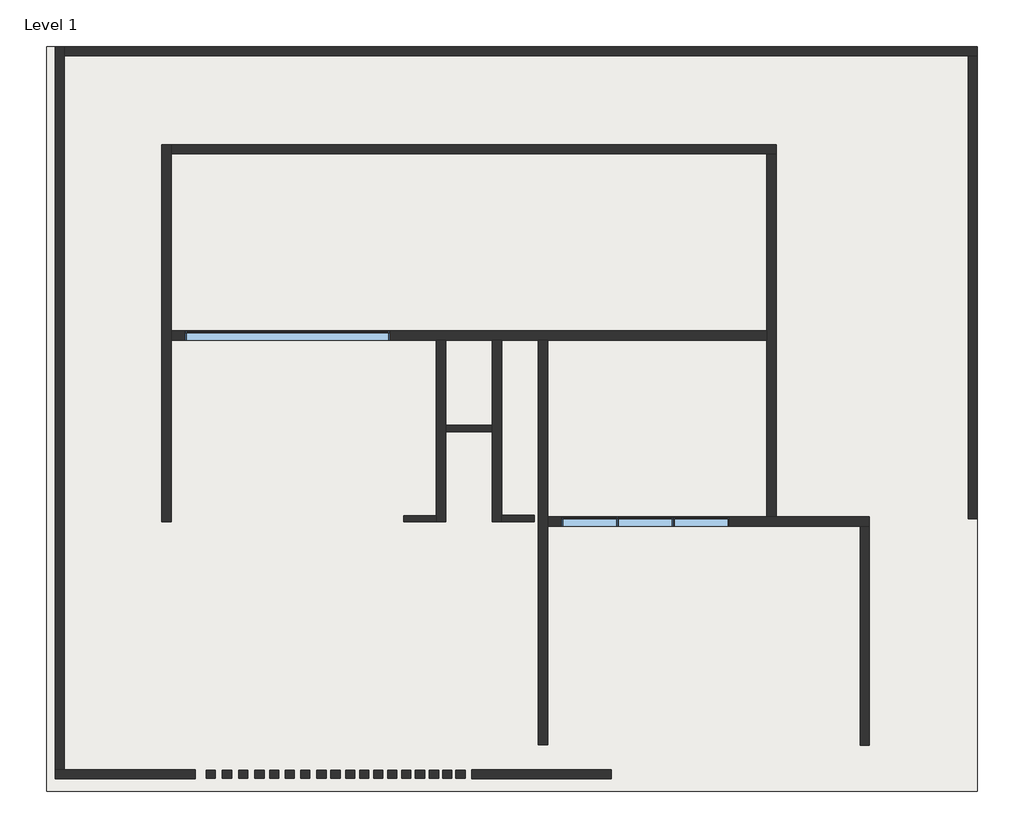
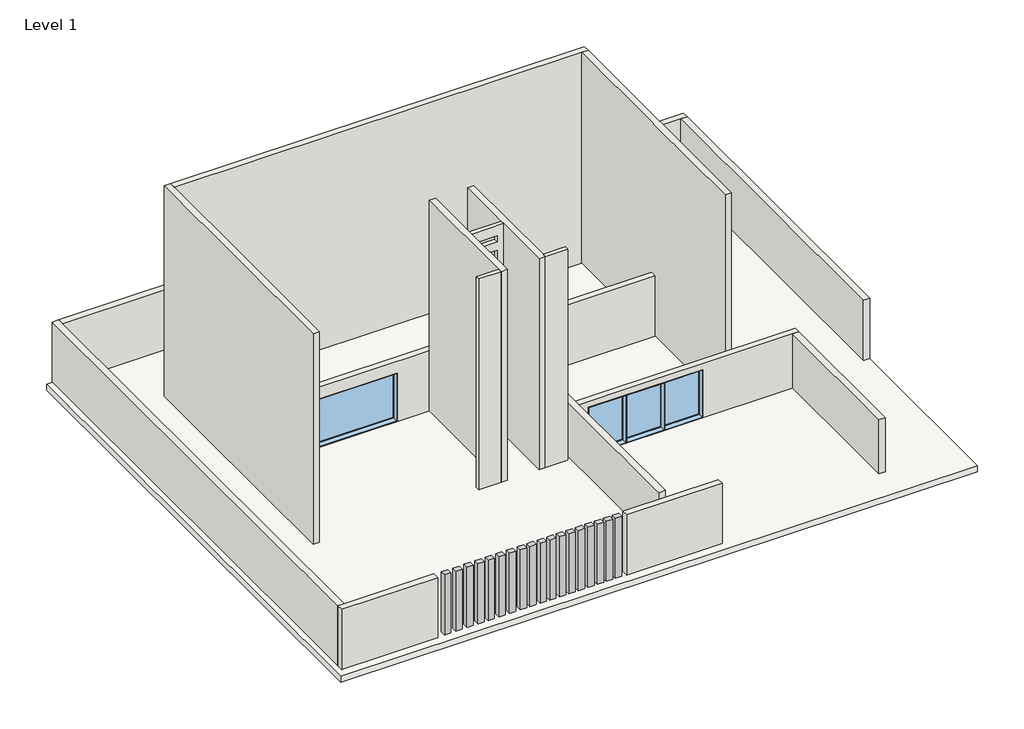
# One storey: 18 columns, 17 walls, 4 windows, 1 slab.
"""IFC4 building model written with IfcOpenShell, lengths in millimetres."""

from ifc_helpers import new_model, si_unit, frame, origin, origin_with_axes, place, context, project, spatial, polyline, outline, extrude, faceted_brep, transform, mapped, element, save
from components import column_263bc08f, window_e4c9328c, window_1de08d8e

model = new_model("IFC4")

# Units and contexts
model_context = context("Model", 3, world=origin())
ifc_project = project(units=[si_unit("LENGTHUNIT", "METRE", prefix="MILLI")], contexts=[model_context])

# Site, building, storey
site = spatial("IfcSite", under=ifc_project)
building = spatial("IfcBuilding", under=site)
storey = spatial("IfcBuildingStorey", under=building, Name="Level 1", Elevation=0.0)

# Columns
placement = place(None, origin())
column_shape = column_263bc08f(model_context)
element("IfcColumn", 1, ObjectType="Rectangular Column : 18\" x 18\"", at=placement, inside=storey, context=model_context, shape_type="MappedRepresentation", body=[
    mapped(column_shape, transform((-8214.6338476, -8321.9583832, 0.0), x_axis=(1.0, 0.0, 0.0), y_axis=(0.0, 1.0, 0.0), z_axis=(0.0, 0.0, 1.0))),
])
element("IfcColumn", 2, ObjectType="Rectangular Column : 18\" x 18\"", at=placement, inside=storey, context=model_context, shape_type="MappedRepresentation", body=[
    mapped(column_shape, transform((-8646.4338476, -8321.9583832, 0.0), x_axis=(1.0, 0.0, 0.0), y_axis=(0.0, 1.0, 0.0), z_axis=(0.0, 0.0, 1.0))),
])
element("IfcColumn", 3, ObjectType="Rectangular Column : 18\" x 18\"", at=placement, inside=storey, context=model_context, shape_type="MappedRepresentation", body=[
    mapped(column_shape, transform((-9078.2338476, -8321.9583832, 0.0), x_axis=(1.0, 0.0, 0.0), y_axis=(0.0, 1.0, 0.0), z_axis=(0.0, 0.0, 1.0))),
])
element("IfcColumn", 4, ObjectType="Rectangular Column : 18\" x 18\"", at=placement, inside=storey, context=model_context, shape_type="MappedRepresentation", body=[
    mapped(column_shape, transform((-9535.4338476, -8321.9583832, 0.0), x_axis=(1.0, 0.0, 0.0), y_axis=(0.0, 1.0, 0.0), z_axis=(0.0, 0.0, 1.0))),
])
element("IfcColumn", 5, ObjectType="Rectangular Column : 18\" x 18\"", at=placement, inside=storey, context=model_context, shape_type="MappedRepresentation", body=[
    mapped(column_shape, transform((-9992.6338476, -8321.9583832, 0.0), x_axis=(1.0, 0.0, 0.0), y_axis=(0.0, 1.0, 0.0), z_axis=(0.0, 0.0, 1.0))),
])
element("IfcColumn", 6, ObjectType="Rectangular Column : 18\" x 18\"", at=placement, inside=storey, context=model_context, shape_type="MappedRepresentation", body=[
    mapped(column_shape, transform((-10449.8338476, -8321.9583832, 0.0), x_axis=(1.0, 0.0, 0.0), y_axis=(0.0, 1.0, 0.0), z_axis=(0.0, 0.0, 1.0))),
])
element("IfcColumn", 7, ObjectType="Rectangular Column : 18\" x 18\"", at=placement, inside=storey, context=model_context, shape_type="MappedRepresentation", body=[
    mapped(column_shape, transform((-10907.0338476, -8321.9583832, 0.0), x_axis=(1.0, 0.0, 0.0), y_axis=(0.0, 1.0, 0.0), z_axis=(0.0, 0.0, 1.0))),
])
element("IfcColumn", 8, ObjectType="Rectangular Column : 18\" x 18\"", at=placement, inside=storey, context=model_context, shape_type="MappedRepresentation", body=[
    mapped(column_shape, transform((-11364.2338476, -8321.9583832, 0.0), x_axis=(1.0, 0.0, 0.0), y_axis=(0.0, 1.0, 0.0), z_axis=(0.0, 0.0, 1.0))),
])
element("IfcColumn", 9, ObjectType="Rectangular Column : 18\" x 18\"", at=placement, inside=storey, context=model_context, shape_type="MappedRepresentation", body=[
    mapped(column_shape, transform((-11821.4338476, -8321.9583832, 0.0), x_axis=(1.0, 0.0, 0.0), y_axis=(0.0, 1.0, 0.0), z_axis=(0.0, 0.0, 1.0))),
])
element("IfcColumn", 10, ObjectType="Rectangular Column : 18\" x 18\"", at=placement, inside=storey, context=model_context, shape_type="MappedRepresentation", body=[
    mapped(column_shape, transform((-12304.0338476, -8321.9583832, 0.0), x_axis=(1.0, 0.0, 0.0), y_axis=(0.0, 1.0, 0.0), z_axis=(0.0, 0.0, 1.0))),
])
element("IfcColumn", 11, ObjectType="Rectangular Column : 18\" x 18\"", at=placement, inside=storey, context=model_context, shape_type="MappedRepresentation", body=[
    mapped(column_shape, transform((-12761.2338476, -8321.9583832, 0.0), x_axis=(1.0, 0.0, 0.0), y_axis=(0.0, 1.0, 0.0), z_axis=(0.0, 0.0, 1.0))),
])
element("IfcColumn", 12, ObjectType="Rectangular Column : 18\" x 18\"", at=placement, inside=storey, context=model_context, shape_type="MappedRepresentation", body=[
    mapped(column_shape, transform((-13294.6338476, -8321.9583832, 0.0), x_axis=(1.0, 0.0, 0.0), y_axis=(0.0, 1.0, 0.0), z_axis=(0.0, 0.0, 1.0))),
])
element("IfcColumn", 13, ObjectType="Rectangular Column : 18\" x 18\"", at=placement, inside=storey, context=model_context, shape_type="MappedRepresentation", body=[
    mapped(column_shape, transform((-13802.6338476, -8321.9583832, 0.0), x_axis=(1.0, 0.0, 0.0), y_axis=(0.0, 1.0, 0.0), z_axis=(0.0, 0.0, 1.0))),
])
element("IfcColumn", 14, ObjectType="Rectangular Column : 18\" x 18\"", at=placement, inside=storey, context=model_context, shape_type="MappedRepresentation", body=[
    mapped(column_shape, transform((-14310.6338476, -8321.9583832, 0.0), x_axis=(1.0, 0.0, 0.0), y_axis=(0.0, 1.0, 0.0), z_axis=(0.0, 0.0, 1.0))),
])
element("IfcColumn", 15, ObjectType="Rectangular Column : 18\" x 18\"", at=placement, inside=storey, context=model_context, shape_type="MappedRepresentation", body=[
    mapped(column_shape, transform((-14793.2338476, -8321.9583832, 0.0), x_axis=(1.0, 0.0, 0.0), y_axis=(0.0, 1.0, 0.0), z_axis=(0.0, 0.0, 1.0))),
])
element("IfcColumn", 16, ObjectType="Rectangular Column : 18\" x 18\"", at=placement, inside=storey, context=model_context, shape_type="MappedRepresentation", body=[
    mapped(column_shape, transform((-15326.6338476, -8321.9583832, 0.0), x_axis=(1.0, 0.0, 0.0), y_axis=(0.0, 1.0, 0.0), z_axis=(0.0, 0.0, 1.0))),
])
element("IfcColumn", 17, ObjectType="Rectangular Column : 18\" x 18\"", at=placement, inside=storey, context=model_context, shape_type="MappedRepresentation", body=[
    mapped(column_shape, transform((-15860.0338476, -8321.9583832, 0.0), x_axis=(1.0, 0.0, 0.0), y_axis=(0.0, 1.0, 0.0), z_axis=(0.0, 0.0, 1.0))),
])
element("IfcColumn", 18, ObjectType="Rectangular Column : 18\" x 18\"", at=placement, inside=storey, context=model_context, shape_type="MappedRepresentation", body=[
    mapped(column_shape, transform((-16393.4338476, -8321.9583832, 0.0), x_axis=(1.0, 0.0, 0.0), y_axis=(0.0, 1.0, 0.0), z_axis=(0.0, 0.0, 1.0))),
])

# Slab
element("IfcSlab", 19, ObjectType="Generic - 12\"", at=placement, inside=storey, context=model_context, shape_type="SweptSolid", body=[
    extrude(outline(polyline([(-21767.9603059, 15503.2416168), (8712.0396941, 15503.2416168), (8712.0396941, -8880.7583832), (-21767.9603059, -8880.7583832), (-21767.9603059, 15503.2416168)])), frame((0.0, 0.0, -304.8), z_axis=(0.0, 0.0, 1.0), x_axis=(1.0, 0.0, 0.0)), (0.0, 0.0, 1.0), 304.8),
])

# Walls
element("IfcWall", 20, ObjectType="Generic - 12\"", at=placement, inside=storey, context=model_context, shape_type="Brep", body=[
    faceted_brep([(-17993.6338476, 12293.8223265, 0.0), (-17993.6338476, -50.5776735, 0.0), (-17993.6338476, -50.5776735, 10668.0), (-17993.6338476, 12293.8223265, 10668.0), (-17688.8338476, 12293.8223265, 0.0), (-17688.8338476, 12293.8223265, 10668.0), (-17688.8338476, 11989.0223265, 10668.0), (-17688.8338476, 6185.1223265, 10668.0), (-17688.8338476, 5880.3223265, 10668.0), (-17688.8338476, -50.5776735, 10668.0), (-17688.8338476, -50.5776735, 0.0), (-17688.8338476, 5893.0223265, 0.0), (-17688.8338476, 6197.8223265, 0.0), (-17688.8338476, 11989.0223265, 0.0)], [[[0, 1, 2, 3]], [[4, 5, 6, 7, 8, 9, 10, 11, 12, 13]], [[1, 0, 4, 13, 12, 11, 10]], [[2, 1, 10, 9]], [[3, 2, 9, 8, 7, 6, 5]], [[0, 3, 5, 4]]]),
])
element("IfcWall", 21, ObjectType="Generic - 12\"", at=placement, inside=storey, context=model_context, shape_type="Brep", body=[
    faceted_brep([(2123.1661524, 12293.8223265, 0.0), (-17688.8338476, 12293.8223265, 0.0), (-17688.8338476, 12293.8223265, 10668.0), (2123.1661524, 12293.8223265, 10668.0), (2123.1661524, 11989.0223265, 0.0), (2123.1661524, 11989.0223265, 10668.0), (1818.3661524, 11989.0223265, 10668.0), (-17688.8338476, 11989.0223265, 10668.0), (-17688.8338476, 11989.0223265, 0.0), (1818.3661524, 11989.0223265, 0.0)], [[[0, 1, 2, 3]], [[4, 5, 6, 7, 8, 9]], [[1, 0, 4, 9, 8]], [[3, 2, 7, 6, 5]], [[0, 3, 5, 4]], [[2, 1, 8, 7]]]),
])
element("IfcWall", 22, ObjectType="Generic - 12\"", at=placement, inside=storey, context=model_context, shape_type="Brep", body=[
    faceted_brep([(2123.1661524, 101.8223265, 0.0), (2123.1661524, 11989.0223265, 0.0), (2123.1661524, 11989.0223265, 10668.0), (2123.1661524, 101.8223265, 10668.0), (1818.3661524, 101.8223265, 0.0), (1818.3661524, 101.8223265, 10668.0), (1818.3661524, 5880.3223265, 10668.0), (1818.3661524, 6185.1223265, 10668.0), (1818.3661524, 11989.0223265, 10668.0), (1818.3661524, 11989.0223265, 0.0), (1818.3661524, 6197.8223265, 0.0), (1818.3661524, 5893.0223265, 0.0)], [[[0, 1, 2, 3]], [[4, 5, 6, 7, 8, 9, 10, 11]], [[1, 0, 4, 11, 10, 9]], [[3, 2, 8, 7, 6, 5]], [[2, 1, 9, 8]], [[0, 3, 5, 4]]]),
])
element("IfcWall", 23, ObjectType="Generic - 12\"", at=placement, inside=storey, context=model_context, shape_type="Brep", body=[
    faceted_brep([(-17688.8338476, 5893.0223265, 0.0), (-9002.0338476, 5893.0223265, 0.0), (-8697.2338476, 5893.0223265, 0.0), (-7173.2338476, 5893.0223265, 0.0), (-6868.4338476, 5893.0223265, 0.0), (-5664.3603059, 5893.0223265, 0.0), (-5359.5603059, 5893.0223265, 0.0), (1818.3661524, 5893.0223265, 0.0), (1818.3661524, 5893.0223265, 3048.0), (-6868.4338476, 5893.0223265, 3048.0), (-7173.2338476, 5893.0223265, 3048.0), (-8697.2338476, 5893.0223265, 3048.0), (-9002.0338476, 5893.0223265, 3048.0), (-17688.8338476, 5893.0223265, 3048.0), (-10526.0338476, 5893.0223265, 2457.3629027), (-10526.0338476, 5893.0223265, 18.9629027), (-17231.6338476, 5893.0223265, 18.9629027), (-17231.6338476, 5893.0223265, 2457.3629027), (1818.3661524, 6197.8223265, 0.0), (-17688.8338476, 6197.8223265, 0.0), (-17688.8338476, 6197.8223265, 3048.0), (1818.3661524, 6197.8223265, 3048.0), (-10526.0338476, 6197.8223265, 18.9629027), (-10526.0338476, 6197.8223265, 2457.3629027), (-17231.6338476, 6197.8223265, 2457.3629027), (-17231.6338476, 6197.8223265, 18.9629027)], [[[0, 1, 2, 3, 4, 5, 6, 7, 8, 9, 10, 11, 12, 13], [14, 15, 16, 17]], [[18, 19, 20, 21], [22, 23, 24, 25]], [[7, 6, 5, 4, 3, 2, 1, 0, 19, 18]], [[13, 12, 11, 10, 9, 8, 21, 20]], [[0, 13, 20, 19]], [[8, 7, 18, 21]], [[14, 23, 22, 15]], [[15, 22, 25, 16]], [[23, 14, 17, 24]], [[24, 17, 16, 25]]]),
])
element("IfcWall", 24, ObjectType="Generic - 12\"", at=placement, inside=storey, context=model_context, shape_type="Brep", body=[
    faceted_brep([(-7173.2338476, 5893.0223265, 0.0), (-7173.2338476, 3099.0223265, 0.0), (-7173.2338476, 2895.8223265, 0.0), (-7173.2338476, -53.7526735, 0.0), (-7173.2338476, -53.7526735, 10668.0), (-7173.2338476, 2895.8223265, 10668.0), (-7173.2338476, 3099.0223265, 10668.0), (-7173.2338476, 5880.3223265, 10668.0), (-7173.2338476, 5880.3223265, 3048.0), (-7173.2338476, 5893.0223265, 3048.0), (-6868.4338476, 5893.0223265, 0.0), (-6868.4338476, 5893.0223265, 3048.0), (-6868.4338476, 5880.3223265, 3048.0), (-6868.4338476, 5880.3223265, 10668.0), (-6868.4338476, 149.4473265, 10668.0), (-6868.4338476, -53.7526735, 10668.0), (-6868.4338476, -53.7526735, 0.0), (-6868.4338476, 149.4473265, 0.0)], [[[0, 1, 2, 3, 4, 5, 6, 7, 8, 9]], [[10, 11, 12, 13, 14, 15, 16, 17]], [[3, 2, 1, 0, 10, 17, 16]], [[7, 6, 5, 4, 15, 14, 13]], [[8, 12, 11, 9]], [[0, 9, 11, 10]], [[7, 13, 12, 8]], [[4, 3, 16, 15]]]),
])
element("IfcWall", 25, ObjectType="Generic - 12\"", at=placement, inside=storey, context=model_context, shape_type="Brep", body=[
    faceted_brep([(-9002.0338476, 5893.0223265, 0.0), (-9002.0338476, 139.9223265, 0.0), (-9002.0338476, -63.2776735, 0.0), (-9002.0338476, -63.2776735, 10668.0), (-9002.0338476, 139.9223265, 10668.0), (-9002.0338476, 5880.3223265, 10668.0), (-9002.0338476, 5880.3223265, 3048.0), (-9002.0338476, 5893.0223265, 3048.0), (-8697.2338476, 5893.0223265, 0.0), (-8697.2338476, 5893.0223265, 3048.0), (-8697.2338476, 5880.3223265, 3048.0), (-8697.2338476, 5880.3223265, 10668.0), (-8697.2338476, 3099.0223265, 10668.0), (-8697.2338476, 2895.8223265, 10668.0), (-8697.2338476, -63.2776735, 10668.0), (-8697.2338476, -63.2776735, 0.0), (-8697.2338476, 2895.8223265, 0.0), (-8697.2338476, 3099.0223265, 0.0)], [[[0, 1, 2, 3, 4, 5, 6, 7]], [[8, 9, 10, 11, 12, 13, 14, 15, 16, 17]], [[2, 1, 0, 8, 17, 16, 15]], [[5, 4, 3, 14, 13, 12, 11]], [[6, 10, 9, 7]], [[0, 7, 9, 8]], [[5, 11, 10, 6]], [[3, 2, 15, 14]]]),
])
element("IfcWall", 26, ObjectType="Generic - 12\"", at=placement, inside=storey, context=model_context, shape_type="Brep", body=[
    faceted_brep([(-5664.3603059, 5893.0223265, 0.0), (-5664.3603059, -7356.7583832, 0.0), (-5664.3603059, -7356.7583832, 2743.2), (-5664.3603059, 5893.0223265, 2743.2), (-5359.5603059, 5893.0223265, 0.0), (-5359.5603059, 5893.0223265, 2743.2), (-5359.5603059, 101.8223265, 2743.2), (-5359.5603059, -202.9776735, 2743.2), (-5359.5603059, -7356.7583832, 2743.2), (-5359.5603059, -7356.7583832, 0.0), (-5359.5603059, -202.9776735, 0.0), (-5359.5603059, 101.8223265, 0.0)], [[[0, 1, 2, 3]], [[4, 5, 6, 7, 8, 9, 10, 11]], [[1, 0, 4, 11, 10, 9]], [[2, 1, 9, 8]], [[3, 2, 8, 7, 6, 5]], [[0, 3, 5, 4]]]),
])
element("IfcWall", 27, ObjectType="Generic - 12\"", at=placement, inside=storey, context=model_context, shape_type="Brep", body=[
    faceted_brep([(5171.1661524, 101.8223265, 0.0), (2123.1661524, 101.8223265, 0.0), (1818.3661524, 101.8223265, 0.0), (-5359.5603059, 101.8223265, 0.0), (-5359.5603059, 101.8223265, 2743.2), (5171.1661524, 101.8223265, 2743.2), (584.0396941, 101.8223265, 2440.70147), (-4902.3603059, 101.8223265, 2440.70147), (-4902.3603059, 101.8223265, 2.30147), (584.0396941, 101.8223265, 2.30147), (-5359.5603059, -202.9776735, 0.0), (4866.3661524, -202.9776735, 0.0), (5171.1661524, -202.9776735, 0.0), (5171.1661524, -202.9776735, 2743.2), (4866.3661524, -202.9776735, 2743.2), (-5359.5603059, -202.9776735, 2743.2), (584.0396941, -202.9776735, 2.30147), (-4902.3603059, -202.9776735, 2.30147), (-4902.3603059, -202.9776735, 2440.70147), (584.0396941, -202.9776735, 2440.70147)], [[[0, 1, 2, 3, 4, 5], [6, 7, 8, 9]], [[10, 11, 12, 13, 14, 15], [16, 17, 18, 19]], [[3, 2, 1, 0, 12, 11, 10]], [[5, 4, 15, 14, 13]], [[4, 3, 10, 15]], [[0, 5, 13, 12]], [[8, 17, 16, 9]], [[18, 17, 8, 7]], [[18, 7, 6, 19]], [[19, 6, 9, 16]]]),
])
element("IfcWall", 28, ObjectType="Generic - 12\"", at=placement, inside=storey, context=model_context, shape_type="SweptSolid", body=[
    extrude(outline(polyline([(4866.3661524, -7365.7776735), (4866.3661524, -202.9776735), (5171.1661524, -202.9776735), (5171.1661524, -7365.7776735), (4866.3661524, -7365.7776735)])), origin_with_axes(), (0.0, 0.0, 1.0), 2743.2),
])
element("IfcWall", 29, ObjectType="Generic - 12\"", at=placement, inside=storey, context=model_context, shape_type="SweptSolid", body=[
    extrude(outline(polyline([(-7848.7603059, -8169.5583832), (-3276.7603059, -8169.5583832), (-3276.7603059, -8474.3583832), (-7848.7603059, -8474.3583832), (-7848.7603059, -8169.5583832)])), origin_with_axes(), (0.0, 0.0, 1.0), 3048.0),
])
element("IfcWall", 30, ObjectType="Generic - 12\"", at=placement, inside=storey, context=model_context, shape_type="Brep", body=[
    faceted_brep([(-16891.1603059, -8169.5583832, 0.0), (-21184.5080121, -8169.5583832, 0.0), (-21489.3080121, -8169.5583832, 0.0), (-21489.3080121, -8169.5583832, 3048.0), (-21184.5080121, -8169.5583832, 3048.0), (-16891.1603059, -8169.5583832, 3048.0), (-16891.1603059, -8474.3583832, 0.0), (-16891.1603059, -8474.3583832, 3048.0), (-21489.3080121, -8474.3583832, 3048.0), (-21489.3080121, -8474.3583832, 0.0)], [[[0, 1, 2, 3, 4, 5]], [[6, 7, 8, 9]], [[2, 1, 0, 6, 9]], [[5, 4, 3, 8, 7]], [[0, 5, 7, 6]], [[3, 2, 9, 8]]]),
])
element("IfcWall", 31, ObjectType="Generic - 12\"", at=placement, inside=storey, context=model_context, shape_type="Brep", body=[
    faceted_brep([(-21184.5080121, -8169.5583832, 0.0), (-21184.5080121, 15198.4416168, 0.0), (-21184.5080121, 15503.2416168, 0.0), (-21184.5080121, 15503.2416168, 3048.0), (-21184.5080121, 15198.4416168, 3048.0), (-21184.5080121, -8169.5583832, 3048.0), (-21489.3080121, -8169.5583832, 0.0), (-21489.3080121, -8169.5583832, 3048.0), (-21489.3080121, 15503.2416168, 3048.0), (-21489.3080121, 15503.2416168, 0.0)], [[[0, 1, 2, 3, 4, 5]], [[6, 7, 8, 9]], [[2, 1, 0, 6, 9]], [[5, 4, 3, 8, 7]], [[0, 5, 7, 6]], [[3, 2, 9, 8]]]),
])
element("IfcWall", 32, ObjectType="Generic - 12\"", at=placement, inside=storey, context=model_context, shape_type="Brep", body=[
    faceted_brep([(-21184.5080121, 15198.4416168, 0.0), (8407.2396941, 15198.4416168, 0.0), (8712.0396941, 15198.4416168, 0.0), (8712.0396941, 15198.4416168, 3048.0), (8407.2396941, 15198.4416168, 3048.0), (-21184.5080121, 15198.4416168, 3048.0), (-21184.5080121, 15503.2416168, 0.0), (-21184.5080121, 15503.2416168, 3048.0), (8712.0396941, 15503.2416168, 3048.0), (8712.0396941, 15503.2416168, 0.0)], [[[0, 1, 2, 3, 4, 5]], [[6, 7, 8, 9]], [[2, 1, 0, 6, 9]], [[5, 4, 3, 8, 7]], [[0, 5, 7, 6]], [[3, 2, 9, 8]]]),
])
element("IfcWall", 33, ObjectType="Generic - 12\"", at=placement, inside=storey, context=model_context, shape_type="SweptSolid", body=[
    extrude(outline(polyline([(8407.2396941, 47.8473265), (8407.2396941, 15198.4416168), (8712.0396941, 15198.4416168), (8712.0396941, 47.8473265), (8407.2396941, 47.8473265)])), origin_with_axes(), (0.0, 0.0, 1.0), 3048.0),
])
element("IfcWall", 34, ObjectType="Generic - 8\"", at=placement, inside=storey, context=model_context, shape_type="SweptSolid", body=[
    extrude(outline(polyline([(0.0, -8697.2338476), (0.0, -7173.2338476), (10668.0, -7173.2338476), (10668.0, -8697.2338476), (0.0, -8697.2338476)]), holes=[polyline([(9426.8097194, -7478.0338476), (6988.4097194, -7478.0338476), (6988.4097194, -8392.4338476), (9426.8097194, -8392.4338476), (9426.8097194, -7478.0338476)]), polyline([(6419.6691739, -7478.0338476), (3981.2691739, -7478.0338476), (3981.2691739, -8392.4338476), (6419.6691739, -8392.4338476), (6419.6691739, -7478.0338476)]), polyline([(10156.6050177, -8392.4338476), (10156.6050177, -7478.0338476), (9851.8050177, -7478.0338476), (9851.8050177, -8392.4338476), (10156.6050177, -8392.4338476)]), polyline([(3431.6251543, -8392.4338476), (3431.6251543, -7478.0338476), (3126.8251543, -7478.0338476), (3126.8251543, -8392.4338476), (3431.6251543, -8392.4338476)])]), frame((0.0, 2895.8223265, 0.0), z_axis=(0.0, 1.0, 0.0), x_axis=(0.0, 0.0, 1.0)), (0.0, 0.0, 1.0), 203.2),
])
element("IfcWall", 35, ObjectType="Generic - 8\" 2", at=placement, inside=storey, context=model_context, shape_type="SweptSolid", body=[
    extrude(outline(polyline([(-5801.6338476, -53.7526735), (-6868.4338476, -53.7526735), (-6868.4338476, 149.4473265), (-5801.6338476, 149.4473265), (-5801.6338476, -53.7526735)])), origin_with_axes(), (0.0, 0.0, 1.0), 10668.0),
])
element("IfcWall", 36, ObjectType="Generic - 8\" 2", at=placement, inside=storey, context=model_context, shape_type="SweptSolid", body=[
    extrude(outline(polyline([(-10068.8338476, 139.9223265), (-9002.0338476, 139.9223265), (-9002.0338476, -63.2776735), (-10068.8338476, -63.2776735), (-10068.8338476, 139.9223265)])), origin_with_axes(), (0.0, 0.0, 1.0), 10668.0),
])

# Windows
window_shape = window_e4c9328c(model_context)
element("IfcWindow", 37, ObjectType="Fixed : 264\" x 96\"", at=placement, inside=storey, context=model_context, shape_type="MappedRepresentation", body=[
    mapped(window_shape, transform((-13840.7338476, 6045.4223265, -285.8370973), x_axis=(1.0, 0.0, 0.0), y_axis=(0.0, 1.0, 0.0), z_axis=(0.0, 0.0, 1.0))),
])
window_2_shape = window_1de08d8e(model_context)
element("IfcWindow", 38, ObjectType="Fixed : 72\" x 96\"", at=placement, inside=storey, context=model_context, shape_type="MappedRepresentation", body=[
    mapped(window_2_shape, transform((-3949.8603059, -50.5776735, -302.49853), x_axis=(1.0, 0.0, 0.0), y_axis=(0.0, 1.0, 0.0), z_axis=(0.0, 0.0, 1.0))),
])
element("IfcWindow", 39, ObjectType="Fixed : 72\" x 96\"", at=placement, inside=storey, context=model_context, shape_type="MappedRepresentation", body=[
    mapped(window_2_shape, transform((-2121.0603059, -50.5776735, -302.49853), x_axis=(1.0, 0.0, 0.0), y_axis=(0.0, 1.0, 0.0), z_axis=(0.0, 0.0, 1.0))),
])
element("IfcWindow", 40, ObjectType="Fixed : 72\" x 96\"", at=placement, inside=storey, context=model_context, shape_type="MappedRepresentation", body=[
    mapped(window_2_shape, transform((-292.2603059, -50.5776735, -302.49853), x_axis=(1.0, 0.0, 0.0), y_axis=(0.0, 1.0, 0.0), z_axis=(0.0, 0.0, 1.0))),
])

save(model, "model.ifc")

# Revit data of these elements
# Type "Rectangular Column : 18\" x 18\""
#   Assembly Code = "B1010200"
#   Depth = 0' - 10"
#   Offset Base = 0' - 0"
#   Offset Top = 0' - 0"
#   Width = 1' - 0"
#   Material = Rigid insulation
# Type "Generic - 12\""
#   Assembly Code = "B1010"
#   Function = 0
#   Layers, outside or top first: 1' - 0" "Concrete Masonry Units" (function 1)
# Type "Generic - 12\""
#   Assembly Code = "B2010"
#   Layers, outside or top first: 1' - 0" "Concrete Masonry Units" (function 1)
# Type "Generic - 8\""
#   Assembly Code = "B2010"
#   Layers, outside or top first: 0' - 8" no material (function 1)
# Type "Generic - 8\" 2"
#   Assembly Code = "B2010"
#   Layers, outside or top first: 0' - 8" "Plywood, Sheathing" (function 1)
# Type "Fixed : 264\" x 96\""
#   Type Mark = "10"
#   Construction Type Id = "GSP4R"
#   Assembly Code = "B2020100"
#   Analytic Construction = "1/8 in Pilkington single glazing"
#   Visual Light Transmittance = 0.9
#   Solar Heat Gain Coefficient = 0.78
#   Heat Transfer Coefficient (U) = 0.6496 BTU/(h·ft²·°F)
#   Height = 8' - 0"
#   Default Sill Height = 1' - 0"
#   Width = 22' - 0"
#   Window Inset = 0' - 0 3/4"
#   Define Thermal Properties by = 1
#   Glass Pane Material = Glass
#   Sash Material = Iron, Ductile
#   Wall Closure = (empty or 0)
# Type "Fixed : 72\" x 96\""
#   Type Mark = "11"
#   Construction Type Id = "GSP4R"
#   Assembly Code = "B2020100"
#   Analytic Construction = "1/8 in Pilkington single glazing"
#   Visual Light Transmittance = 0.9
#   Solar Heat Gain Coefficient = 0.78
#   Heat Transfer Coefficient (U) = 0.6496 BTU/(h·ft²·°F)
#   Height = 8' - 0"
#   Default Sill Height = 1' - 0"
#   Width = 6' - 0"
#   Window Inset = 0' - 0 3/4"
#   Define Thermal Properties by = 1
#   Glass Pane Material = Glass
#   Sash Material = Iron, Ductile
#   Wall Closure = (empty or 0)
# Elements 1, 2, 3, 4, 5, 6, 7, 8, 9, 10, 11, 12, 13, 14, 15, 16, 17, 18 (IfcColumn, "Rectangular Column : 18\" x 18\"")
#   Phase Created = New Construction
#   Materials on its faces: "Rigid insulation"
# Element 19 (IfcSlab, "Generic - 12\"")
#   built-in parameter 1001955 = 3.14159 (stored number, unit not read)
#   Height Offset From Level = 0' - 0"
#   Phase Created = New Construction
#   Materials on its faces: "Concrete Masonry Units"
# Elements 20, 21, 22 (IfcWall, "Generic - 12\"")
#   Top Offset = 0' - 0"
#   Base Offset = 0' - 0"
#   Unconnected Height = 35' - 0"
#   wall height = 35' - 0"
#   Phase Created = New Construction
#   Base Constraint = Level 1
#   Materials on its faces: "Concrete Masonry Units"
# Elements 23, 29, 30, 31, 32, 33 (IfcWall, "Generic - 12\"")
#   Top Offset = 0' - 0"
#   Base Offset = 0' - 0"
#   Unconnected Height = 10' - 0"
#   wall height = 10' - 0"
#   Phase Created = New Construction
#   Base Constraint = Level 1
#   Materials on its faces: "Concrete Masonry Units"
# Elements 24, 25 (IfcWall, "Generic - 12\"")
#   Top Offset = 0' - 0"
#   Base Offset = 0' - 0"
#   Unconnected Height = 35' - 0"
#   wall height = 35' - 0"
#   Phase Created = New Construction
#   Base Constraint = Level 1
#   Materials on its faces: "Concrete Masonry Units", "Plywood, Sheathing"
# Elements 26, 27, 28 (IfcWall, "Generic - 12\"")
#   Top Offset = 0' - 0"
#   Base Offset = 0' - 0"
#   Unconnected Height = 9' - 0"
#   wall height = 9' - 0"
#   Phase Created = New Construction
#   Base Constraint = Level 1
#   Materials on its faces: "Concrete Masonry Units"
# Element 34 (IfcWall, "Generic - 8\"")
#   Top Offset = 0' - 0"
#   Base Offset = 0' - 0"
#   Unconnected Height = 35' - 0"
#   wall height = 35' - 0"
#   Phase Created = New Construction
#   Base Constraint = Level 1
#   Materials on its faces: "Default Wall"
# Elements 35, 36 (IfcWall, "Generic - 8\" 2")
#   Top Offset = 0' - 0"
#   Base Offset = 0' - 0"
#   Unconnected Height = 35' - 0"
#   wall height = 35' - 0"
#   Phase Created = New Construction
#   Base Constraint = Level 1
#   Materials on its faces: "Plywood, Sheathing"
# Element 37 (IfcWindow, "Fixed : 264\" x 96\"")
#   Mark = "1"
#   Phase Created = New Construction
#   Materials on its faces: "Iron, Ductile", "Glass"
# Element 38 (IfcWindow, "Fixed : 72\" x 96\"")
#   Mark = "2"
#   Phase Created = New Construction
#   Materials on its faces: "Iron, Ductile", "Glass"
# Element 39 (IfcWindow, "Fixed : 72\" x 96\"")
#   Mark = "3"
#   Phase Created = New Construction
#   Materials on its faces: "Iron, Ductile", "Glass"
# Element 40 (IfcWindow, "Fixed : 72\" x 96\"")
#   Mark = "4"
#   Phase Created = New Construction
#   Materials on its faces: "Iron, Ductile", "Glass"
# Materials
#   "Rigid insulation": class "Generic", colour RGB 127 127 127, transparency 0, Description = "Rigid foam insulation board", Cost = 0
#   "Concrete Masonry Units": class "Masonry", colour RGB 227 227 227, transparency 0, Description = "Concrete masonry units", Cost = 0
#   "Plywood, Sheathing": class "Wood", colour RGB 212 179 113, transparency 0, Description = "Plywood, sheathing grade", Cost = 0
#   "Glass": class "Glass", colour RGB 0 128 192, transparency 0.75, Description = "Soda Lime Glass", Cost = 0
#   "Iron, Ductile": class "Metal", colour RGB 0 0 0, transparency 0, Description = "Ductile cast iron", Cost = 0
#   "Default Wall": colour RGB 128 128 128, transparency 0
